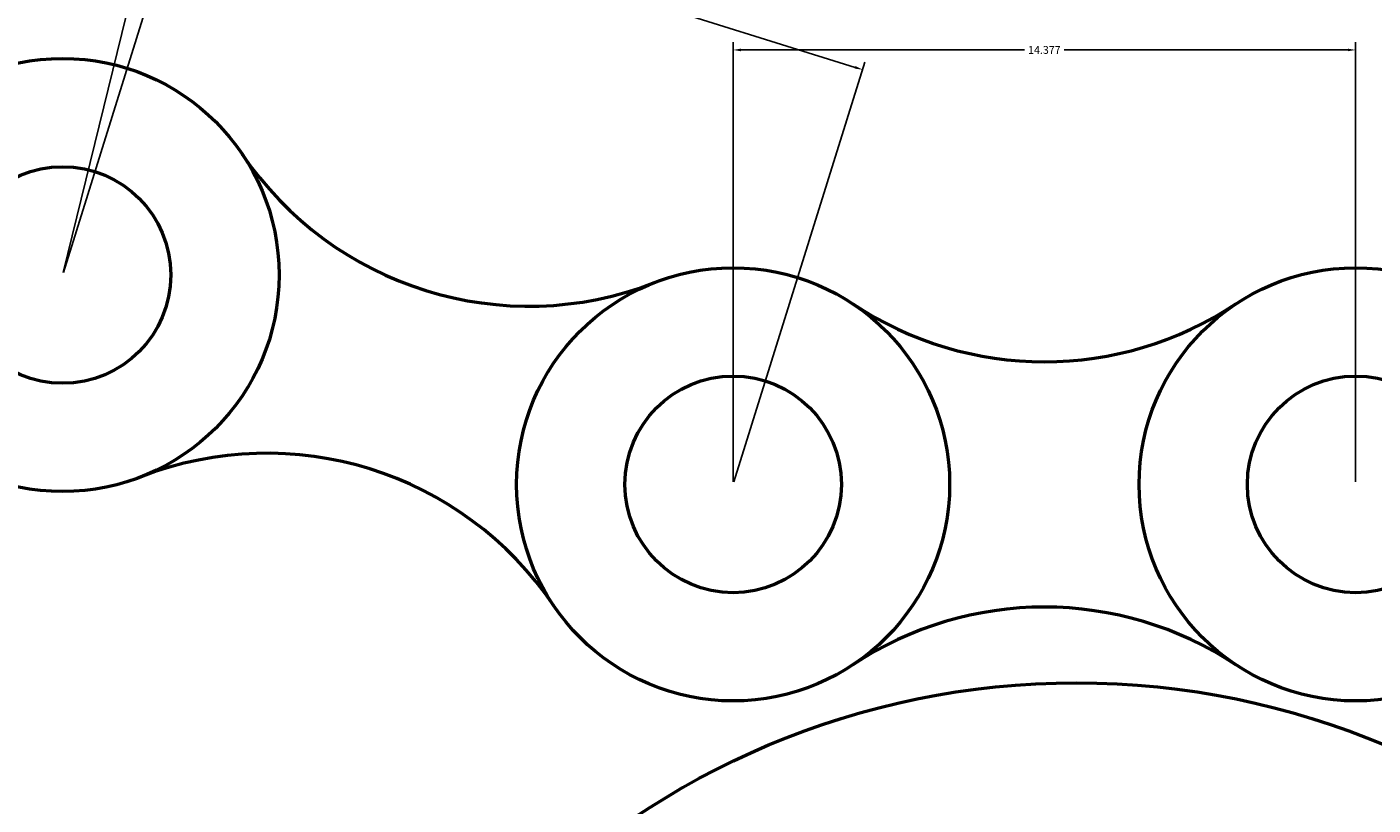
# Model space of a CAD drawing. Units: inches. Extents: x 413 to 622, y 326 to 447.
# Tile 13 of 15: x 568 to 600, y 402 to 420. Entities that reach past the tile are written whole.
import ezdxf

# ---------------------------------------------------------------- set-up
doc = ezdxf.new("R2010")
doc.units = ezdxf.units.IN
doc.header["$MEASUREMENT"] = 0
doc.layers.add('M-DIMS', color=2, linetype='Continuous', lineweight=18)
doc.layers.add('M-OUTL', color=7, linetype='Continuous', lineweight=50)
doc.styles.get("Standard").update_dxf_attribs({"font": 'arial.ttf'})
doc.dimstyles.get("Standard").update_dxf_attribs({"dimtxt": 0.18, "dimasz": 0.18, "dimexe": 0.18, "dimexo": 0.0625, "dimgap": 0.09, "dimtad": 0, "dimtih": 1, "dimtoh": 1, "dimdec": 4, "dimzin": 0, "dimdsep": 46, "dimtxsty": 'Standard', "dimcen": 0.09, "dimadec": 0, "dimazin": 0, "dimtfac": 1, "dimtdec": 4, "dimtofl": 0, "dimtmove": 0, "dimatfit": 3, "dimfxl": 1, "dimtolj": 1, "dimtzin": 0, "dimarcsym": 0})

# ---------------------------------------------------------------- blocks, each defined once
blk = doc.blocks.new('CHAIN-ROLLER-PIN')
for radius in [5, 2.5]:
    blk.add_circle((5, 5), radius)
blk = doc.blocks.new('*D11')
at = {"layer": 'Defpoints', "color": 0, "transparency": 16777216}
for p in [(621.66, 446.422), (621.66, 388.074), (423.314, 378.888)]:
    blk.add_point(p, dxfattribs=at)
at = {"layer": 'M-DIMS', "color": 0, "lineweight": -2, "transparency": 16777216}
for p, q in [((423.314, 378.95), (423.314, 446.602)), ((621.66, 388.137), (621.66, 446.602)), ((423.494, 446.422), (522.031, 446.422)), ((621.48, 446.422), (522.943, 446.422))]:
    blk.add_line(p, q, dxfattribs=at)
at = {"layer": 'M-DIMS', "color": 0, "transparency": 16777216}
for points in [[(423.494, 446.452), (423.494, 446.392), (423.314, 446.422)], [(621.48, 446.452), (621.48, 446.392), (621.66, 446.422)]]:
    blk.add_solid(points, dxfattribs=at)
at = {"layer": 'M-DIMS', "color": 0, "transparency": 16777216, "insert": (522.487, 446.422), "char_height": 0.18, "attachment_point": 5}
blk.add_mtext('\\A1;198.35', dxfattribs=at)
blk = doc.blocks.new('*D21')
at = {"layer": 'Defpoints', "color": 0, "transparency": 16777216}
for p in [(571.652, 423.827), (549.452, 418.938), (569.266, 414.085)]:
    blk.add_point(p, dxfattribs=at)
at = {"layer": 'M-DIMS', "color": 0, "lineweight": -2, "transparency": 16777216}
for p, q in [((549.467, 418.998), (551.881, 428.855)), ((552.013, 428.637), (561.421, 426.333)), ((571.478, 423.87), (562.07, 426.174)), ((569.281, 414.145), (571.695, 424.002))]:
    blk.add_line(p, q, dxfattribs=at)
at = {"layer": 'M-DIMS', "color": 0, "transparency": 16777216}
for points in [[(552.02, 428.666), (552.006, 428.608), (551.838, 428.68)], [(571.485, 423.899), (571.47, 423.841), (571.652, 423.827)]]:
    blk.add_solid(points, dxfattribs=at)
at = {"layer": 'M-DIMS', "color": 0, "transparency": 16777216, "insert": (561.745, 426.254), "char_height": 0.18, "attachment_point": 5}
blk.add_mtext('\\A1;20.4', dxfattribs=at)
blk = doc.blocks.new('*D22')
at = {"layer": 'Defpoints', "color": 0, "transparency": 16777216}
for p in [(587.742, 418.825), (569.266, 414.085), (584.753, 409.25)]:
    blk.add_point(p, dxfattribs=at)
at = {"layer": 'M-DIMS', "color": 0, "lineweight": -2, "transparency": 16777216}
for p, q in [((569.285, 414.144), (572.309, 423.831)), ((572.427, 423.606), (579.543, 421.384)), ((587.57, 418.879), (580.454, 421.1)), ((584.771, 409.31), (587.795, 418.997))]:
    blk.add_line(p, q, dxfattribs=at)
at = {"layer": 'M-DIMS', "color": 0, "transparency": 16777216}
for points in [[(572.436, 423.635), (572.418, 423.577), (572.255, 423.66)], [(587.579, 418.907), (587.561, 418.85), (587.742, 418.825)]]:
    blk.add_solid(points, dxfattribs=at)
at = {"layer": 'M-DIMS', "color": 0, "transparency": 16777216, "insert": (579.999, 421.242), "char_height": 0.18, "attachment_point": 5}
blk.add_mtext('\\A1;16.223', dxfattribs=at)
blk = doc.blocks.new('*D23')
at = {"layer": 'Defpoints', "color": 0, "transparency": 16777216}
for p in [(599.13, 419.281), (584.753, 409.25), (599.13, 409.25)]:
    blk.add_point(p, dxfattribs=at)
at = {"layer": 'M-DIMS', "color": 0, "lineweight": -2, "transparency": 16777216}
for p, q in [((584.753, 409.313), (584.753, 419.461)), ((599.13, 409.313), (599.13, 419.461)), ((584.933, 419.281), (591.486, 419.281)), ((598.95, 419.281), (592.396, 419.281))]:
    blk.add_line(p, q, dxfattribs=at)
at = {"layer": 'M-DIMS', "color": 0, "transparency": 16777216}
for points in [[(584.933, 419.311), (584.933, 419.251), (584.753, 419.281)], [(598.95, 419.311), (598.95, 419.251), (599.13, 419.281)]]:
    blk.add_solid(points, dxfattribs=at)
at = {"layer": 'M-DIMS', "color": 0, "transparency": 16777216, "insert": (591.941, 419.281), "char_height": 0.18, "attachment_point": 5}
blk.add_mtext('\\A1;14.377', dxfattribs=at)

msp = doc.modelspace()

# ---------------------------------------------------------------- linework, layer by layer
at = {"layer": 'M-OUTL'}
msp.add_circle((592.6836, 386.3915), 18.28, dxfattribs=at)
for centre, start, end in [((580.0367, 421.3648), 214.05585, 291.27039), ((591.9411, 420.0821), 236.43016, 303.56984), ((573.9824, 401.9704), 34.05585, 111.27039), ((591.9411, 398.4186), 56.43016, 123.56984)]:
    msp.add_arc(centre, 8, start, end, dxfattribs=at)

# ---------------------------------------------------------------- block references
for p in [(564.2668, 409.0853), (579.7532, 404.2509), (594.1299, 404.2509)]:
    msp.add_blockref('CHAIN-ROLLER-PIN', p, dxfattribs=at)

# ---------------------------------------------------------------- dimensions: what is measured, and where the dimension line sits
at = {"layer": 'M-DIMS'}
for base, p1, p2, override, picture, middle in [((621.66, 446.422), (423.3136, 378.8878), (621.66, 388.0741), {"dimdec": 2, "dimlfac": 1, "dimrnd": 0, "dimzin": 0, "dimdsep": 46, "dimlunit": 2}, '*D11', (522.4868, 446.422)), ((599.1295, 419.2809), (584.7527, 409.2504), (599.1295, 409.2504), {"dimdec": 3, "dimlfac": 1, "dimrnd": 0, "dimzin": 0, "dimdsep": 46, "dimlunit": 2}, '*D23', (591.9411, 419.2809))]:
    dim = msp.add_linear_dim(base=base, p1=p1, p2=p2, dimstyle='Standard', override=override, dxfattribs=at)
    dim.commit()
    dim.dimension.update_dxf_attribs({"geometry": picture, "text_midpoint": middle})
for base, p1, p2, angle, override, picture, middle in [((571.6524, 423.8274), (549.4524, 418.9375), (569.2663, 414.0848), 346.23831, {"dimdec": 1, "dimlfac": 1, "dimrnd": 0, "dimzin": 0, "dimdsep": 46, "dimlunit": 2}, '*D21', (561.7455, 426.2537)), ((587.7417, 418.8252), (569.2663, 414.0848), (584.7527, 409.2504), 342.66312, {"dimdec": 3, "dimlfac": 1, "dimrnd": 0, "dimzin": 0, "dimdsep": 46, "dimlunit": 2}, '*D22', (579.9985, 421.2424))]:
    dim = msp.add_linear_dim(base=base, p1=p1, p2=p2, angle=angle, dimstyle='Standard', override=override, dxfattribs=at)
    dim.commit()
    dim.dimension.update_dxf_attribs({"geometry": picture, "text_midpoint": middle})

doc.saveas('drawing.dxf')
